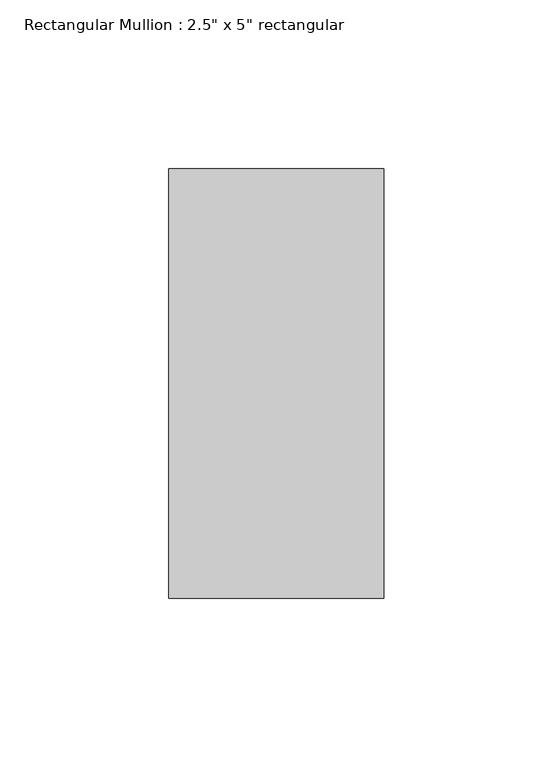
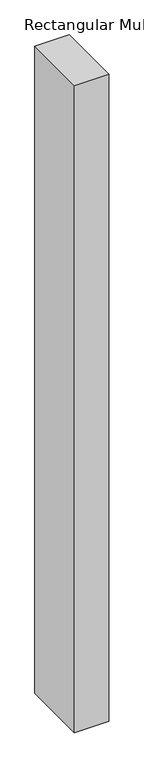
"""IFC4 building model written with IfcOpenShell, lengths in millimetres: member geometry."""

from ifc_helpers import new_model, si_unit, frame, origin, place, context, project, spatial, polyline, outline, extrude, source, transform, mapped, element, save


def member_ab7d1daf(model_context):
    return source(origin(), model_context, "Body", "SweptSolid", [
        extrude(outline(polyline([(0.0, 63.5), (0.0, -63.5), (-63.5, -63.5), (-63.5, 63.5), (0.0, 63.5)])), frame((0.0, 0.0, -1270.0), z_axis=(0.0, 0.0, 1.0), x_axis=(1.0, 0.0, 0.0)), (0.0, 0.0, 1.0), 1270.0),
    ])


if __name__ == "__main__":
    model = new_model("IFC4")
    model_context = context("Model", 3, world=origin())
    ifc_project = project(units=[si_unit("LENGTHUNIT", "METRE", prefix="MILLI")], contexts=[model_context])
    site = spatial("IfcSite", under=ifc_project)
    building = spatial("IfcBuilding", under=site)
    placement = place(None, origin())
    member_shape = member_ab7d1daf(model_context)
    element("IfcMember", 1, ObjectType="Rectangular Mullion : 2.5\" x 5\" rectangular", at=placement, inside=building, context=model_context, shape_type="MappedRepresentation", body=[
        mapped(member_shape, transform((0.0, 0.0, 0.0), x_axis=(1.0, 0.0, 0.0), y_axis=(0.0, 1.0, 0.0), z_axis=(0.0, 0.0, 1.0))),
    ])
    save(model, "model.ifc")

# Revit data of these elements
# Type "Rectangular Mullion : 2.5\" x 5\" rectangular"
#   built-in parameter 1007304 = 0.416667 (stored number, unit not read)
#   built-in parameter 1007301 = 0.104167 (stored number, unit not read)
#   built-in parameter 1007300 = 0.104167 (stored number, unit not read)
